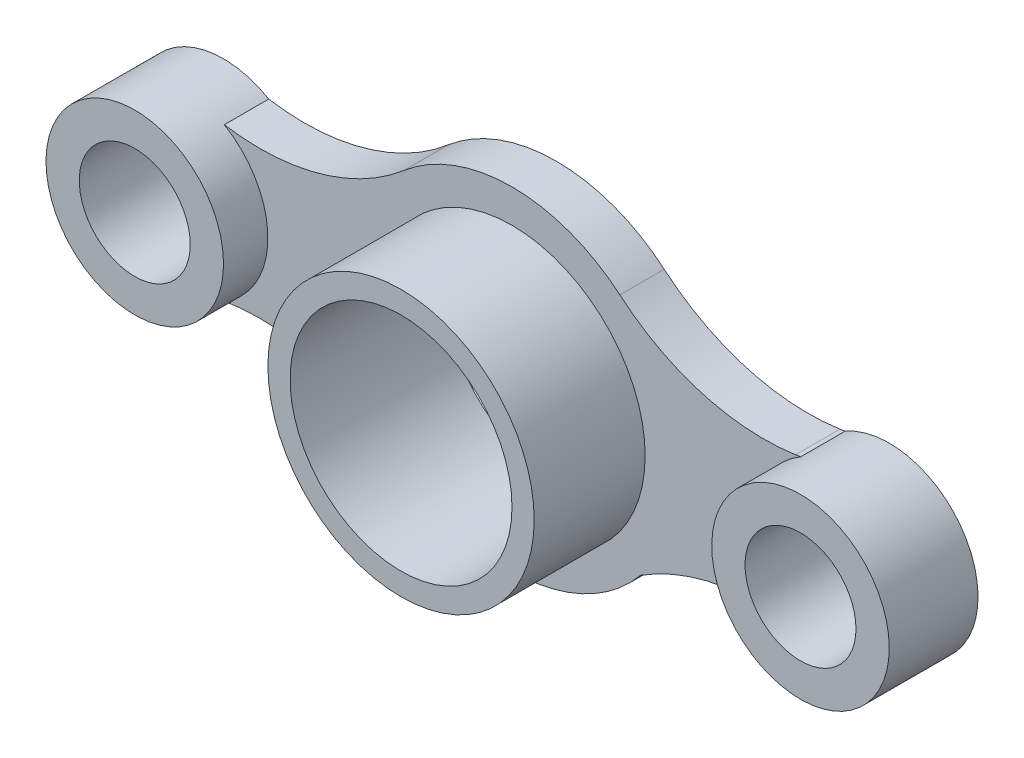
ISO-10303-21;
HEADER;
FILE_DESCRIPTION(('STEP AP214'),'2;1');
FILE_NAME('part.step','',(''),(''),'','','');
FILE_SCHEMA(('AUTOMOTIVE_DESIGN { 1 0 10303 214 1 1 1 1 }'));
ENDSEC;
DATA;
#1=APPLICATION_CONTEXT('core data for automotive mechanical design processes');
#2=APPLICATION_PROTOCOL_DEFINITION('international standard','automotive_design',2000,#1);
#3=PRODUCT_CONTEXT('',#1,'mechanical');
#4=PRODUCT('Part','Part','',(#3));
#5=PRODUCT_RELATED_PRODUCT_CATEGORY('part','',(#4));
#6=PRODUCT_DEFINITION_FORMATION('','',#4);
#7=PRODUCT_DEFINITION_CONTEXT('part definition',#1,'design');
#8=PRODUCT_DEFINITION('design','',#6,#7);
#9=PRODUCT_DEFINITION_SHAPE('','',#8);
#10=(LENGTH_UNIT() NAMED_UNIT(*) SI_UNIT(.MILLI.,.METRE.));
#11=(NAMED_UNIT(*) PLANE_ANGLE_UNIT() SI_UNIT($,.RADIAN.));
#12=(NAMED_UNIT(*) SI_UNIT($,.STERADIAN.) SOLID_ANGLE_UNIT());
#13=UNCERTAINTY_MEASURE_WITH_UNIT(LENGTH_MEASURE(1.E-05),#10,'distance_accuracy_value','');
#14=(GEOMETRIC_REPRESENTATION_CONTEXT(3) GLOBAL_UNCERTAINTY_ASSIGNED_CONTEXT((#13)) GLOBAL_UNIT_ASSIGNED_CONTEXT((#10,
#11,#12)) REPRESENTATION_CONTEXT('',''));
#15=CARTESIAN_POINT('',(0.,0.,0.));
#16=DIRECTION('',(0.,0.,1.));
#17=DIRECTION('',(1.,0.,0.));
#18=AXIS2_PLACEMENT_3D('',#15,#16,#17);
#19=CARTESIAN_POINT('',(0.,0.,20.));
#20=DIRECTION('',(0.,0.,1.));
#21=DIRECTION('',(1.,0.,0.));
#22=AXIS2_PLACEMENT_3D('',#19,#20,#21);
#23=PLANE('',#22);
#24=CARTESIAN_POINT('',(0.,0.,20.));
#25=DIRECTION('',(0.,0.,1.));
#26=DIRECTION('',(1.,0.,0.));
#27=AXIS2_PLACEMENT_3D('',#24,#25,#26);
#28=CIRCLE('',#27,60.);
#29=CARTESIAN_POINT('',(60.,0.,20.));
#30=VERTEX_POINT('',#29);
#31=EDGE_CURVE('E254',#30,#30,#28,.T.);
#32=ORIENTED_EDGE('',*,*,#31,.F.);
#33=EDGE_LOOP('',(#32));
#34=FACE_BOUND('',#33,.T.);
#35=CARTESIAN_POINT('',(111.786103262779,-132.522528747727,20.));
#36=DIRECTION('',(0.,0.,1.));
#37=DIRECTION('',(1.,0.,0.));
#38=AXIS2_PLACEMENT_3D('',#35,#36,#37);
#39=CIRCLE('',#38,100.54);
#40=CARTESIAN_POINT('',(127.784288058385,-33.2635257140185,20.));
#41=VERTEX_POINT('',#40);
#42=CARTESIAN_POINT('',(57.94980163206,-47.6111383061243,20.));
#43=VERTEX_POINT('',#42);
#44=EDGE_CURVE('E164',#41,#43,#39,.T.);
#45=ORIENTED_EDGE('',*,*,#44,.F.);
#46=CARTESIAN_POINT('',(150.,0.,20.));
#47=DIRECTION('',(0.,0.,1.));
#48=DIRECTION('',(1.,0.,0.));
#49=AXIS2_PLACEMENT_3D('',#46,#47,#48);
#50=CIRCLE('',#49,40.);
#51=CARTESIAN_POINT('',(130.089258317401,34.6923963664781,20.));
#52=VERTEX_POINT('',#51);
#53=EDGE_CURVE('E184',#52,#41,#50,.T.);
#54=ORIENTED_EDGE('',*,*,#53,.F.);
#55=CARTESIAN_POINT('',(112.106622021826,142.151771778757,20.));
#56=DIRECTION('',(0.,0.,1.));
#57=DIRECTION('',(1.,0.,0.));
#58=AXIS2_PLACEMENT_3D('',#55,#56,#57);
#59=CIRCLE('',#58,108.953625787011);
#60=CARTESIAN_POINT('',(127.784288058385,34.3319991960708,20.));
#61=VERTEX_POINT('',#60);
#62=EDGE_CURVE('E240',#61,#52,#59,.T.);
#63=ORIENTED_EDGE('',*,*,#62,.F.);
#64=CARTESIAN_POINT('',(113.394986258363,133.291324141767,20.));
#65=DIRECTION('',(0.,0.,1.));
#66=DIRECTION('',(1.,0.,0.));
#67=AXIS2_PLACEMENT_3D('',#64,#65,#66);
#68=CIRCLE('',#67,100.);
#69=CARTESIAN_POINT('',(48.5978512535842,57.1248532036144,20.));
#70=VERTEX_POINT('',#69);
#71=EDGE_CURVE('E262',#61,#70,#68,.F.);
#72=ORIENTED_EDGE('',*,*,#71,.T.);
#73=CARTESIAN_POINT('',(0.,0.,20.));
#74=DIRECTION('',(0.,0.,1.));
#75=DIRECTION('',(1.,0.,0.));
#76=AXIS2_PLACEMENT_3D('',#73,#74,#75);
#77=CIRCLE('',#76,75.);
#78=CARTESIAN_POINT('',(-48.6771910753612,57.0572613171433,20.));
#79=VERTEX_POINT('',#78);
#80=EDGE_CURVE('E136',#70,#79,#77,.T.);
#81=ORIENTED_EDGE('',*,*,#80,.T.);
#82=CARTESIAN_POINT('',(-113.580112509176,133.133609740001,20.));
#83=DIRECTION('',(0.,0.,1.));
#84=DIRECTION('',(1.,0.,0.));
#85=AXIS2_PLACEMENT_3D('',#82,#83,#84);
#86=CIRCLE('',#85,100.);
#87=CARTESIAN_POINT('',(-129.642270947794,34.4320035408477,20.));
#88=VERTEX_POINT('',#87);
#89=EDGE_CURVE('E123',#88,#79,#86,.T.);
#90=ORIENTED_EDGE('',*,*,#89,.F.);
#91=CARTESIAN_POINT('',(-150.,0.,20.));
#92=DIRECTION('',(0.,0.,1.));
#93=DIRECTION('',(1.,0.,0.));
#94=AXIS2_PLACEMENT_3D('',#91,#92,#93);
#95=CIRCLE('',#94,40.);
#96=CARTESIAN_POINT('',(-129.642270947794,-34.4320035408477,20.));
#97=VERTEX_POINT('',#96);
#98=EDGE_CURVE('E11',#88,#97,#95,.F.);
#99=ORIENTED_EDGE('',*,*,#98,.T.);
#100=CARTESIAN_POINT('',(-113.484125045025,-133.117941348546,20.));
#101=DIRECTION('',(0.,0.,1.));
#102=DIRECTION('',(1.,0.,0.));
#103=AXIS2_PLACEMENT_3D('',#100,#101,#102);
#104=CIRCLE('',#103,100.);
#105=CARTESIAN_POINT('',(-50.5482093328372,-55.4064845775625,20.));
#106=VERTEX_POINT('',#105);
#107=EDGE_CURVE('E125',#97,#106,#104,.F.);
#108=ORIENTED_EDGE('',*,*,#107,.T.);
#109=CARTESIAN_POINT('',(0.,0.,20.));
#110=DIRECTION('',(0.,0.,1.));
#111=DIRECTION('',(1.,0.,0.));
#112=AXIS2_PLACEMENT_3D('',#109,#110,#111);
#113=CIRCLE('',#112,75.);
#114=EDGE_CURVE('E62',#106,#43,#113,.T.);
#115=ORIENTED_EDGE('',*,*,#114,.T.);
#116=EDGE_LOOP('',(#45,#54,#63,#72,#81,#90,#99,#108,#115));
#117=FACE_BOUND('',#116,.T.);
#118=ADVANCED_FACE('F50',(#34,#117),#23,.T.);
#119=CARTESIAN_POINT('',(111.786103262779,-132.522528747727,20.));
#120=DIRECTION('',(0.,0.,-1.));
#121=DIRECTION('',(-1.,0.,0.));
#122=AXIS2_PLACEMENT_3D('',#119,#120,#121);
#123=CYLINDRICAL_SURFACE('',#122,100.54);
#124=CARTESIAN_POINT('',(111.786103262779,-132.522528747727,0.));
#125=DIRECTION('',(0.,0.,1.));
#126=DIRECTION('',(1.,0.,0.));
#127=AXIS2_PLACEMENT_3D('',#124,#125,#126);
#128=CIRCLE('',#127,100.54);
#129=CARTESIAN_POINT('',(127.784288058385,-33.2635257140185,0.));
#130=VERTEX_POINT('',#129);
#131=CARTESIAN_POINT('',(57.94980163206,-47.6111383061243,0.));
#132=VERTEX_POINT('',#131);
#133=EDGE_CURVE('E141',#130,#132,#128,.T.);
#134=ORIENTED_EDGE('',*,*,#133,.F.);
#135=DIRECTION('',(0.,0.,-1.));
#136=VECTOR('',#135,1.);
#137=CARTESIAN_POINT('',(127.784288058385,-33.2635257140185,20.));
#138=LINE('',#137,#136);
#139=EDGE_CURVE('E57',#41,#130,#138,.T.);
#140=ORIENTED_EDGE('',*,*,#139,.F.);
#141=ORIENTED_EDGE('',*,*,#44,.T.);
#142=DIRECTION('',(0.,0.,-1.));
#143=VECTOR('',#142,1.);
#144=CARTESIAN_POINT('',(57.94980163206,-47.6111383061243,20.));
#145=LINE('',#144,#143);
#146=EDGE_CURVE('E102',#43,#132,#145,.T.);
#147=ORIENTED_EDGE('',*,*,#146,.T.);
#148=EDGE_LOOP('',(#134,#140,#141,#147));
#149=FACE_BOUND('',#148,.T.);
#150=ADVANCED_FACE('F47',(#149),#123,.F.);
#151=CARTESIAN_POINT('',(150.,0.,20.));
#152=DIRECTION('',(0.,0.,-1.));
#153=DIRECTION('',(-1.,0.,0.));
#154=AXIS2_PLACEMENT_3D('',#151,#152,#153);
#155=CYLINDRICAL_SURFACE('',#154,40.);
#156=CARTESIAN_POINT('',(150.,0.,0.));
#157=DIRECTION('',(0.,0.,1.));
#158=DIRECTION('',(1.,0.,0.));
#159=AXIS2_PLACEMENT_3D('',#156,#157,#158);
#160=CIRCLE('',#159,40.);
#161=CARTESIAN_POINT('',(130.089258317401,34.6923963664781,0.));
#162=VERTEX_POINT('',#161);
#163=EDGE_CURVE('E148',#130,#162,#160,.T.);
#164=ORIENTED_EDGE('',*,*,#163,.T.);
#165=DIRECTION('',(0.,0.,-1.));
#166=VECTOR('',#165,1.);
#167=CARTESIAN_POINT('',(130.089258317401,34.6923963664781,20.));
#168=LINE('',#167,#166);
#169=EDGE_CURVE('E177',#52,#162,#168,.T.);
#170=ORIENTED_EDGE('',*,*,#169,.F.);
#171=ORIENTED_EDGE('',*,*,#53,.T.);
#172=ORIENTED_EDGE('',*,*,#139,.T.);
#173=EDGE_LOOP('',(#164,#170,#171,#172));
#174=FACE_BOUND('',#173,.T.);
#175=CARTESIAN_POINT('',(150.,0.,40.));
#176=DIRECTION('',(0.,0.,1.));
#177=DIRECTION('',(1.,0.,0.));
#178=AXIS2_PLACEMENT_3D('',#175,#176,#177);
#179=CIRCLE('',#178,40.);
#180=CARTESIAN_POINT('',(190.,0.,40.));
#181=VERTEX_POINT('',#180);
#182=EDGE_CURVE('E236',#181,#181,#179,.T.);
#183=ORIENTED_EDGE('',*,*,#182,.F.);
#184=EDGE_LOOP('',(#183));
#185=FACE_BOUND('',#184,.T.);
#186=ADVANCED_FACE('F178',(#174,#185),#155,.T.);
#187=CARTESIAN_POINT('',(112.106622021826,142.151771778757,20.));
#188=DIRECTION('',(0.,0.,-1.));
#189=DIRECTION('',(-1.,0.,0.));
#190=AXIS2_PLACEMENT_3D('',#187,#188,#189);
#191=CYLINDRICAL_SURFACE('',#190,108.953625787011);
#192=CARTESIAN_POINT('',(112.106622021826,142.151771778757,0.));
#193=DIRECTION('',(0.,0.,1.));
#194=DIRECTION('',(1.,0.,0.));
#195=AXIS2_PLACEMENT_3D('',#192,#193,#194);
#196=CIRCLE('',#195,108.953625787011);
#197=CARTESIAN_POINT('',(127.784288058385,34.3319991960708,0.));
#198=VERTEX_POINT('',#197);
#199=EDGE_CURVE('E147',#198,#162,#196,.T.);
#200=ORIENTED_EDGE('',*,*,#199,.F.);
#201=DIRECTION('',(0.,0.,-1.));
#202=VECTOR('',#201,1.);
#203=CARTESIAN_POINT('',(127.784288058385,34.3319991960708,20.));
#204=LINE('',#203,#202);
#205=EDGE_CURVE('E172',#61,#198,#204,.T.);
#206=ORIENTED_EDGE('',*,*,#205,.F.);
#207=ORIENTED_EDGE('',*,*,#62,.T.);
#208=ORIENTED_EDGE('',*,*,#169,.T.);
#209=EDGE_LOOP('',(#200,#206,#207,#208));
#210=FACE_BOUND('',#209,.T.);
#211=ADVANCED_FACE('F198',(#210),#191,.F.);
#212=CARTESIAN_POINT('',(113.394986258363,133.291324141767,20.));
#213=DIRECTION('',(0.,0.,-1.));
#214=DIRECTION('',(-1.,0.,0.));
#215=AXIS2_PLACEMENT_3D('',#212,#213,#214);
#216=CYLINDRICAL_SURFACE('',#215,100.);
#217=CARTESIAN_POINT('',(113.394986258363,133.291324141767,0.));
#218=DIRECTION('',(0.,0.,1.));
#219=DIRECTION('',(1.,0.,0.));
#220=AXIS2_PLACEMENT_3D('',#217,#218,#219);
#221=CIRCLE('',#220,100.);
#222=CARTESIAN_POINT('',(48.5978512535842,57.1248532036144,0.));
#223=VERTEX_POINT('',#222);
#224=EDGE_CURVE('E153',#198,#223,#221,.F.);
#225=ORIENTED_EDGE('',*,*,#224,.T.);
#226=DIRECTION('',(0.,0.,-1.));
#227=VECTOR('',#226,1.);
#228=CARTESIAN_POINT('',(48.5978512535842,57.1248532036144,20.));
#229=LINE('',#228,#227);
#230=EDGE_CURVE('E173',#70,#223,#229,.T.);
#231=ORIENTED_EDGE('',*,*,#230,.F.);
#232=ORIENTED_EDGE('',*,*,#71,.F.);
#233=ORIENTED_EDGE('',*,*,#205,.T.);
#234=EDGE_LOOP('',(#225,#231,#232,#233));
#235=FACE_BOUND('',#234,.T.);
#236=ADVANCED_FACE('F221',(#235),#216,.F.);
#237=CARTESIAN_POINT('',(0.,0.,20.));
#238=DIRECTION('',(0.,0.,-1.));
#239=DIRECTION('',(-1.,0.,0.));
#240=AXIS2_PLACEMENT_3D('',#237,#238,#239);
#241=CYLINDRICAL_SURFACE('',#240,75.);
#242=CARTESIAN_POINT('',(0.,0.,0.));
#243=DIRECTION('',(0.,0.,1.));
#244=DIRECTION('',(1.,0.,0.));
#245=AXIS2_PLACEMENT_3D('',#242,#243,#244);
#246=CIRCLE('',#245,75.);
#247=CARTESIAN_POINT('',(-48.6771910753612,57.0572613171433,0.));
#248=VERTEX_POINT('',#247);
#249=EDGE_CURVE('E154',#223,#248,#246,.T.);
#250=ORIENTED_EDGE('',*,*,#249,.T.);
#251=DIRECTION('',(0.,0.,-1.));
#252=VECTOR('',#251,1.);
#253=CARTESIAN_POINT('',(-48.6771910753612,57.0572613171433,20.));
#254=LINE('',#253,#252);
#255=EDGE_CURVE('E166',#79,#248,#254,.T.);
#256=ORIENTED_EDGE('',*,*,#255,.F.);
#257=ORIENTED_EDGE('',*,*,#80,.F.);
#258=ORIENTED_EDGE('',*,*,#230,.T.);
#259=EDGE_LOOP('',(#250,#256,#257,#258));
#260=FACE_BOUND('',#259,.T.);
#261=ADVANCED_FACE('F219',(#260),#241,.T.);
#262=CARTESIAN_POINT('',(-113.580112509176,133.133609740001,20.));
#263=DIRECTION('',(0.,0.,-1.));
#264=DIRECTION('',(-1.,0.,0.));
#265=AXIS2_PLACEMENT_3D('',#262,#263,#264);
#266=CYLINDRICAL_SURFACE('',#265,100.);
#267=CARTESIAN_POINT('',(-113.580112509176,133.133609740001,0.));
#268=DIRECTION('',(0.,0.,1.));
#269=DIRECTION('',(1.,0.,0.));
#270=AXIS2_PLACEMENT_3D('',#267,#268,#269);
#271=CIRCLE('',#270,100.);
#272=CARTESIAN_POINT('',(-129.642270947793,34.4320035408477,0.));
#273=VERTEX_POINT('',#272);
#274=EDGE_CURVE('E158',#273,#248,#271,.T.);
#275=ORIENTED_EDGE('',*,*,#274,.F.);
#276=DIRECTION('',(0.,0.,-1.));
#277=VECTOR('',#276,1.);
#278=CARTESIAN_POINT('',(-129.642270947793,34.4320035408477,20.));
#279=LINE('',#278,#277);
#280=EDGE_CURVE('E131',#88,#273,#279,.T.);
#281=ORIENTED_EDGE('',*,*,#280,.F.);
#282=ORIENTED_EDGE('',*,*,#89,.T.);
#283=ORIENTED_EDGE('',*,*,#255,.T.);
#284=EDGE_LOOP('',(#275,#281,#282,#283));
#285=FACE_BOUND('',#284,.T.);
#286=ADVANCED_FACE('F220',(#285),#266,.F.);
#287=CARTESIAN_POINT('',(-150.,0.,20.));
#288=DIRECTION('',(0.,0.,-1.));
#289=DIRECTION('',(-1.,0.,0.));
#290=AXIS2_PLACEMENT_3D('',#287,#288,#289);
#291=CYLINDRICAL_SURFACE('',#290,40.);
#292=CARTESIAN_POINT('',(-150.,0.,0.));
#293=DIRECTION('',(0.,0.,1.));
#294=DIRECTION('',(1.,0.,0.));
#295=AXIS2_PLACEMENT_3D('',#292,#293,#294);
#296=CIRCLE('',#295,40.);
#297=CARTESIAN_POINT('',(-129.642270947794,-34.4320035408477,0.));
#298=VERTEX_POINT('',#297);
#299=EDGE_CURVE('E135',#273,#298,#296,.T.);
#300=ORIENTED_EDGE('',*,*,#299,.T.);
#301=DIRECTION('',(0.,0.,-1.));
#302=VECTOR('',#301,1.);
#303=CARTESIAN_POINT('',(-129.642270947794,-34.4320035408477,20.));
#304=LINE('',#303,#302);
#305=EDGE_CURVE('E126',#97,#298,#304,.T.);
#306=ORIENTED_EDGE('',*,*,#305,.F.);
#307=ORIENTED_EDGE('',*,*,#98,.F.);
#308=ORIENTED_EDGE('',*,*,#280,.T.);
#309=EDGE_LOOP('',(#300,#306,#307,#308));
#310=FACE_BOUND('',#309,.T.);
#311=CARTESIAN_POINT('',(-150.,0.,40.));
#312=DIRECTION('',(0.,0.,1.));
#313=DIRECTION('',(1.,0.,0.));
#314=AXIS2_PLACEMENT_3D('',#311,#312,#313);
#315=CIRCLE('',#314,40.);
#316=CARTESIAN_POINT('',(-110.,0.,40.));
#317=VERTEX_POINT('',#316);
#318=EDGE_CURVE('E245',#317,#317,#315,.T.);
#319=ORIENTED_EDGE('',*,*,#318,.F.);
#320=EDGE_LOOP('',(#319));
#321=FACE_BOUND('',#320,.T.);
#322=ADVANCED_FACE('F129',(#310,#321),#291,.T.);
#323=CARTESIAN_POINT('',(-113.484125045025,-133.117941348546,20.));
#324=DIRECTION('',(0.,0.,-1.));
#325=DIRECTION('',(-1.,0.,0.));
#326=AXIS2_PLACEMENT_3D('',#323,#324,#325);
#327=CYLINDRICAL_SURFACE('',#326,100.);
#328=CARTESIAN_POINT('',(-113.484125045025,-133.117941348546,0.));
#329=DIRECTION('',(0.,0.,1.));
#330=DIRECTION('',(1.,0.,0.));
#331=AXIS2_PLACEMENT_3D('',#328,#329,#330);
#332=CIRCLE('',#331,100.);
#333=CARTESIAN_POINT('',(-50.5482093328372,-55.4064845775625,0.));
#334=VERTEX_POINT('',#333);
#335=EDGE_CURVE('E100',#298,#334,#332,.F.);
#336=ORIENTED_EDGE('',*,*,#335,.T.);
#337=DIRECTION('',(0.,0.,-1.));
#338=VECTOR('',#337,1.);
#339=CARTESIAN_POINT('',(-50.5482093328372,-55.4064845775625,20.));
#340=LINE('',#339,#338);
#341=EDGE_CURVE('E132',#106,#334,#340,.T.);
#342=ORIENTED_EDGE('',*,*,#341,.F.);
#343=ORIENTED_EDGE('',*,*,#107,.F.);
#344=ORIENTED_EDGE('',*,*,#305,.T.);
#345=EDGE_LOOP('',(#336,#342,#343,#344));
#346=FACE_BOUND('',#345,.T.);
#347=ADVANCED_FACE('F137',(#346),#327,.F.);
#348=CARTESIAN_POINT('',(0.,0.,20.));
#349=DIRECTION('',(0.,0.,-1.));
#350=DIRECTION('',(-1.,0.,0.));
#351=AXIS2_PLACEMENT_3D('',#348,#349,#350);
#352=CYLINDRICAL_SURFACE('',#351,75.);
#353=CARTESIAN_POINT('',(0.,0.,0.));
#354=DIRECTION('',(0.,0.,1.));
#355=DIRECTION('',(1.,0.,0.));
#356=AXIS2_PLACEMENT_3D('',#353,#354,#355);
#357=CIRCLE('',#356,75.);
#358=EDGE_CURVE('E162',#334,#132,#357,.T.);
#359=ORIENTED_EDGE('',*,*,#358,.T.);
#360=ORIENTED_EDGE('',*,*,#146,.F.);
#361=ORIENTED_EDGE('',*,*,#114,.F.);
#362=ORIENTED_EDGE('',*,*,#341,.T.);
#363=EDGE_LOOP('',(#359,#360,#361,#362));
#364=FACE_BOUND('',#363,.T.);
#365=ADVANCED_FACE('F207',(#364),#352,.T.);
#366=CARTESIAN_POINT('',(0.,0.,0.));
#367=DIRECTION('',(0.,0.,1.));
#368=DIRECTION('',(1.,0.,0.));
#369=AXIS2_PLACEMENT_3D('',#366,#367,#368);
#370=PLANE('',#369);
#371=CARTESIAN_POINT('',(-150.,0.,0.));
#372=DIRECTION('',(0.,0.,1.));
#373=DIRECTION('',(1.,0.,0.));
#374=AXIS2_PLACEMENT_3D('',#371,#372,#373);
#375=CIRCLE('',#374,25.);
#376=CARTESIAN_POINT('',(-125.,0.,0.));
#377=VERTEX_POINT('',#376);
#378=EDGE_CURVE('E239',#377,#377,#375,.T.);
#379=ORIENTED_EDGE('',*,*,#378,.T.);
#380=EDGE_LOOP('',(#379));
#381=FACE_BOUND('',#380,.T.);
#382=CARTESIAN_POINT('',(150.,0.,0.));
#383=DIRECTION('',(0.,0.,1.));
#384=DIRECTION('',(1.,0.,0.));
#385=AXIS2_PLACEMENT_3D('',#382,#383,#384);
#386=CIRCLE('',#385,25.);
#387=CARTESIAN_POINT('',(175.,0.,0.));
#388=VERTEX_POINT('',#387);
#389=EDGE_CURVE('E310',#388,#388,#386,.T.);
#390=ORIENTED_EDGE('',*,*,#389,.T.);
#391=EDGE_LOOP('',(#390));
#392=FACE_BOUND('',#391,.T.);
#393=CARTESIAN_POINT('',(0.,0.,0.));
#394=DIRECTION('',(0.,0.,1.));
#395=DIRECTION('',(1.,0.,0.));
#396=AXIS2_PLACEMENT_3D('',#393,#394,#395);
#397=CIRCLE('',#396,50.);
#398=CARTESIAN_POINT('',(50.,0.,0.));
#399=VERTEX_POINT('',#398);
#400=EDGE_CURVE('E252',#399,#399,#397,.T.);
#401=ORIENTED_EDGE('',*,*,#400,.T.);
#402=EDGE_LOOP('',(#401));
#403=FACE_BOUND('',#402,.T.);
#404=ORIENTED_EDGE('',*,*,#133,.T.);
#405=ORIENTED_EDGE('',*,*,#358,.F.);
#406=ORIENTED_EDGE('',*,*,#335,.F.);
#407=ORIENTED_EDGE('',*,*,#299,.F.);
#408=ORIENTED_EDGE('',*,*,#274,.T.);
#409=ORIENTED_EDGE('',*,*,#249,.F.);
#410=ORIENTED_EDGE('',*,*,#224,.F.);
#411=ORIENTED_EDGE('',*,*,#199,.T.);
#412=ORIENTED_EDGE('',*,*,#163,.F.);
#413=EDGE_LOOP('',(#404,#405,#406,#407,#408,#409,#410,#411,#412));
#414=FACE_BOUND('',#413,.T.);
#415=ADVANCED_FACE('F188',(#381,#392,#403,#414),#370,.F.);
#416=CARTESIAN_POINT('',(0.,0.,70.));
#417=DIRECTION('',(0.,0.,-1.));
#418=DIRECTION('',(-1.,0.,0.));
#419=AXIS2_PLACEMENT_3D('',#416,#417,#418);
#420=CYLINDRICAL_SURFACE('',#419,60.);
#421=CARTESIAN_POINT('',(0.,0.,70.));
#422=DIRECTION('',(0.,0.,1.));
#423=DIRECTION('',(1.,0.,0.));
#424=AXIS2_PLACEMENT_3D('',#421,#422,#423);
#425=CIRCLE('',#424,60.);
#426=CARTESIAN_POINT('',(60.,0.,70.));
#427=VERTEX_POINT('',#426);
#428=EDGE_CURVE('E150',#427,#427,#425,.T.);
#429=ORIENTED_EDGE('',*,*,#428,.F.);
#430=EDGE_LOOP('',(#429));
#431=FACE_BOUND('',#430,.T.);
#432=ORIENTED_EDGE('',*,*,#31,.T.);
#433=EDGE_LOOP('',(#432));
#434=FACE_BOUND('',#433,.T.);
#435=ADVANCED_FACE('F202',(#431,#434),#420,.T.);
#436=CARTESIAN_POINT('',(0.,0.,70.));
#437=DIRECTION('',(0.,0.,1.));
#438=DIRECTION('',(1.,0.,0.));
#439=AXIS2_PLACEMENT_3D('',#436,#437,#438);
#440=PLANE('',#439);
#441=CARTESIAN_POINT('',(0.,0.,70.));
#442=DIRECTION('',(0.,0.,1.));
#443=DIRECTION('',(1.,0.,0.));
#444=AXIS2_PLACEMENT_3D('',#441,#442,#443);
#445=CIRCLE('',#444,50.);
#446=CARTESIAN_POINT('',(50.,0.,70.));
#447=VERTEX_POINT('',#446);
#448=EDGE_CURVE('E253',#447,#447,#445,.T.);
#449=ORIENTED_EDGE('',*,*,#448,.F.);
#450=EDGE_LOOP('',(#449));
#451=FACE_BOUND('',#450,.T.);
#452=ORIENTED_EDGE('',*,*,#428,.T.);
#453=EDGE_LOOP('',(#452));
#454=FACE_BOUND('',#453,.T.);
#455=ADVANCED_FACE('F275',(#451,#454),#440,.T.);
#456=CARTESIAN_POINT('',(0.,0.,0.));
#457=DIRECTION('',(0.,0.,1.));
#458=DIRECTION('',(1.,0.,0.));
#459=AXIS2_PLACEMENT_3D('',#456,#457,#458);
#460=CYLINDRICAL_SURFACE('',#459,50.);
#461=ORIENTED_EDGE('',*,*,#400,.F.);
#462=EDGE_LOOP('',(#461));
#463=FACE_BOUND('',#462,.T.);
#464=ORIENTED_EDGE('',*,*,#448,.T.);
#465=EDGE_LOOP('',(#464));
#466=FACE_BOUND('',#465,.T.);
#467=ADVANCED_FACE('F280',(#463,#466),#460,.F.);
#468=CARTESIAN_POINT('',(-150.,0.,40.));
#469=DIRECTION('',(0.,0.,1.));
#470=DIRECTION('',(1.,0.,0.));
#471=AXIS2_PLACEMENT_3D('',#468,#469,#470);
#472=PLANE('',#471);
#473=CARTESIAN_POINT('',(-150.,0.,40.));
#474=DIRECTION('',(0.,0.,1.));
#475=DIRECTION('',(1.,0.,0.));
#476=AXIS2_PLACEMENT_3D('',#473,#474,#475);
#477=CIRCLE('',#476,25.);
#478=CARTESIAN_POINT('',(-125.,0.,40.));
#479=VERTEX_POINT('',#478);
#480=EDGE_CURVE('E244',#479,#479,#477,.T.);
#481=ORIENTED_EDGE('',*,*,#480,.F.);
#482=EDGE_LOOP('',(#481));
#483=FACE_BOUND('',#482,.T.);
#484=ORIENTED_EDGE('',*,*,#318,.T.);
#485=EDGE_LOOP('',(#484));
#486=FACE_BOUND('',#485,.T.);
#487=ADVANCED_FACE('F282',(#483,#486),#472,.T.);
#488=CARTESIAN_POINT('',(150.,0.,40.));
#489=DIRECTION('',(0.,0.,1.));
#490=DIRECTION('',(1.,0.,0.));
#491=AXIS2_PLACEMENT_3D('',#488,#489,#490);
#492=PLANE('',#491);
#493=CARTESIAN_POINT('',(150.,0.,40.));
#494=DIRECTION('',(0.,0.,1.));
#495=DIRECTION('',(1.,0.,0.));
#496=AXIS2_PLACEMENT_3D('',#493,#494,#495);
#497=CIRCLE('',#496,25.);
#498=CARTESIAN_POINT('',(175.,0.,40.));
#499=VERTEX_POINT('',#498);
#500=EDGE_CURVE('E315',#499,#499,#497,.T.);
#501=ORIENTED_EDGE('',*,*,#500,.F.);
#502=EDGE_LOOP('',(#501));
#503=FACE_BOUND('',#502,.T.);
#504=ORIENTED_EDGE('',*,*,#182,.T.);
#505=EDGE_LOOP('',(#504));
#506=FACE_BOUND('',#505,.T.);
#507=ADVANCED_FACE('F292',(#503,#506),#492,.T.);
#508=CARTESIAN_POINT('',(150.,0.,0.));
#509=DIRECTION('',(0.,0.,1.));
#510=DIRECTION('',(1.,0.,0.));
#511=AXIS2_PLACEMENT_3D('',#508,#509,#510);
#512=CYLINDRICAL_SURFACE('',#511,25.);
#513=ORIENTED_EDGE('',*,*,#389,.F.);
#514=EDGE_LOOP('',(#513));
#515=FACE_BOUND('',#514,.T.);
#516=ORIENTED_EDGE('',*,*,#500,.T.);
#517=EDGE_LOOP('',(#516));
#518=FACE_BOUND('',#517,.T.);
#519=ADVANCED_FACE('F293',(#515,#518),#512,.F.);
#520=CARTESIAN_POINT('',(-150.,0.,0.));
#521=DIRECTION('',(0.,0.,1.));
#522=DIRECTION('',(1.,0.,0.));
#523=AXIS2_PLACEMENT_3D('',#520,#521,#522);
#524=CYLINDRICAL_SURFACE('',#523,25.);
#525=ORIENTED_EDGE('',*,*,#378,.F.);
#526=EDGE_LOOP('',(#525));
#527=FACE_BOUND('',#526,.T.);
#528=ORIENTED_EDGE('',*,*,#480,.T.);
#529=EDGE_LOOP('',(#528));
#530=FACE_BOUND('',#529,.T.);
#531=ADVANCED_FACE('F297',(#527,#530),#524,.F.);
#532=CLOSED_SHELL('',(#118,#150,#186,#211,#236,#261,#286,#322,#347,#365,#415,#435,#455,#467,
#487,#507,#519,#531));
#533=MANIFOLD_SOLID_BREP('B2',#532);
#534=ADVANCED_BREP_SHAPE_REPRESENTATION('',(#18,#533),#14);
#535=SHAPE_DEFINITION_REPRESENTATION(#9,#534);
ENDSEC;
END-ISO-10303-21;
